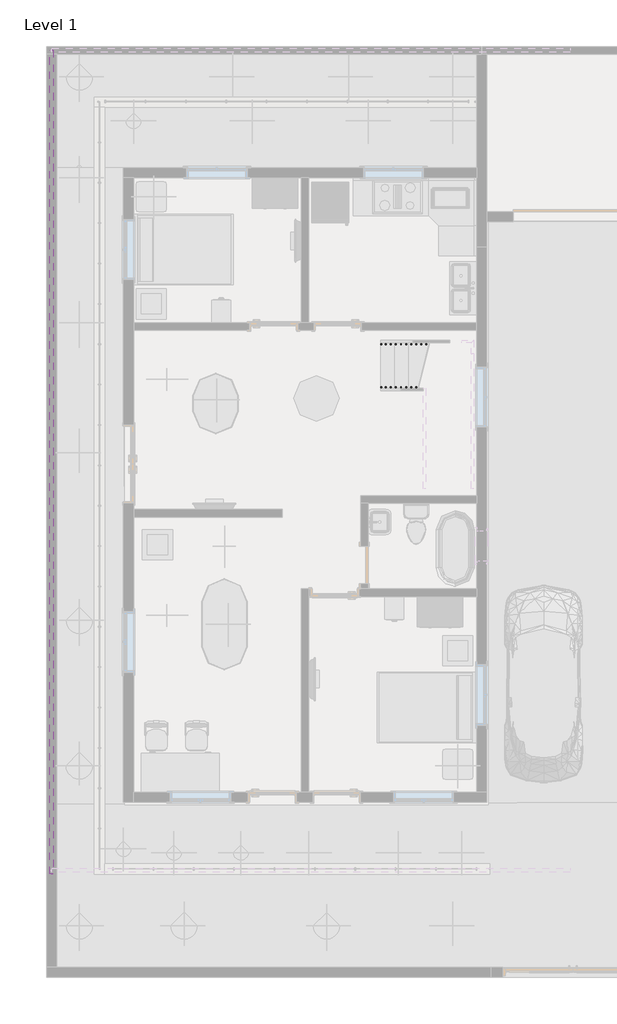
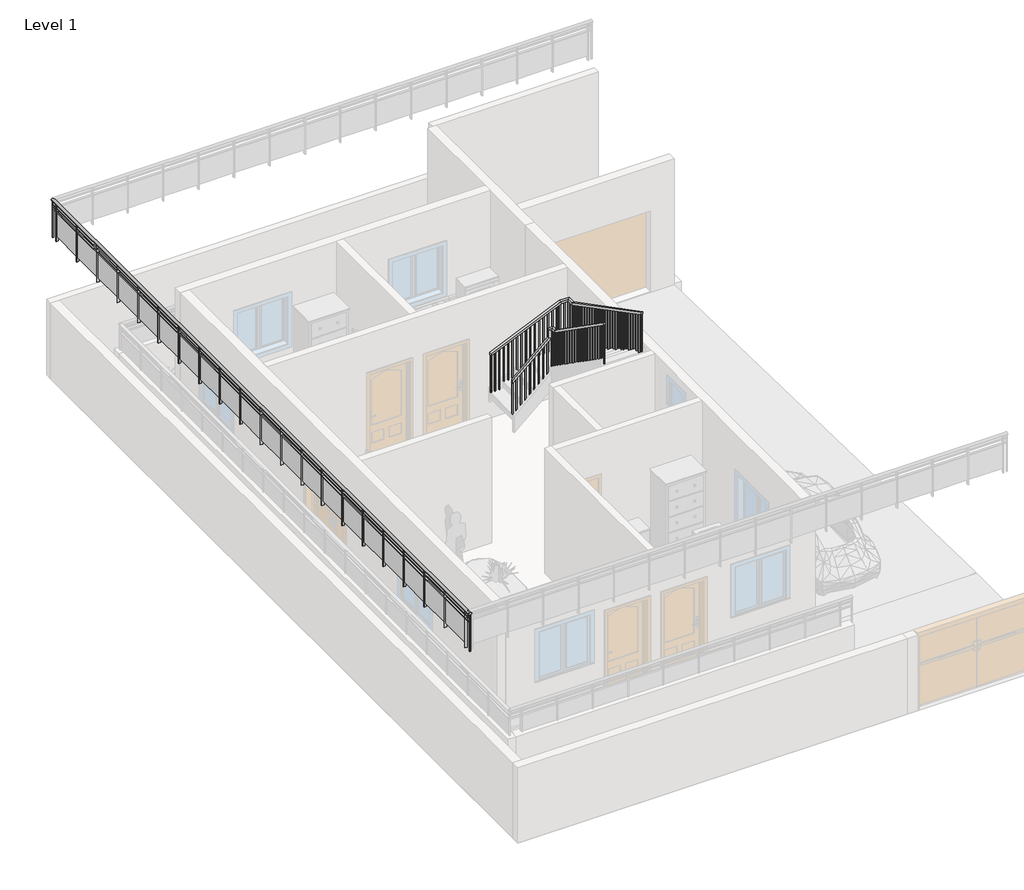
# One storey, part 3 of 5: 3 railings.
"""IFC4 building model written with IfcOpenShell, lengths in millimetres."""

from ifc_helpers import new_model, si_unit, point, frame, origin, place, context, project, spatial, polyline, ellipse_curve, trimmed, outline, extrude, faceted_brep, element, save
from ifc_brep_helpers import plane_surface, extruded_surface, advanced_brep

model = new_model("IFC4")

# Units and contexts
model_context = context("Model", 3, world=origin())
ifc_project = project(units=[si_unit("LENGTHUNIT", "METRE", prefix="MILLI")], contexts=[model_context])

# Site, building, storey
site = spatial("IfcSite", under=ifc_project)
building = spatial("IfcBuilding", under=site)
storey = spatial("IfcBuildingStorey", under=building, Name="Level 1", Elevation=0.0)

# Railings
placement = place(None, origin())
element("IfcRailing", 1, ObjectType="Glass Panel - Bottom Fill", at=placement, inside=storey, context=model_context, shape_type="SolidModel", body=[
    advanced_brep(
    [(-10998.0350785, 11610.9033005, 4267.2), (-11074.2350785, 11610.9033005, 4267.2), (-10998.0350785, -4975.2966995, 4267.2), (-11074.2350785, -4975.2966995, 4267.2)],
    [
        (0, 1, ellipse_curve(frame((-11036.1350785, 11610.9033005, 4267.2), z_axis=(0.0, 1.0, 0.0), x_axis=(-1.0, 0.0, 0.0)), 38.1, 28.575)),
        (1, 0, ellipse_curve(frame((-11036.1350785, 11610.9033005, 4267.2), z_axis=(0.0, 1.0, 0.0), x_axis=(-1.0, 0.0, 0.0)), 38.1, 28.575)),
        (2, 3, ellipse_curve(frame((-11036.1350785, -4975.2966995, 4267.2), z_axis=(0.0, -1.0, 0.0), x_axis=(-1.0, 0.0, 0.0)), 38.1, 28.575)),
        (3, 2, ellipse_curve(frame((-11036.1350785, -4975.2966995, 4267.2), z_axis=(0.0, -1.0, 0.0), x_axis=(-1.0, 0.0, 0.0)), 38.1, 28.575)),
        (0, 2),
        (3, 1),
    ],
    [
        plane_surface(frame((-11036.1350785, 11610.9033005, 4267.2), z_axis=(0.0, 1.0, 0.0), x_axis=(0.0, 0.0, -1.0))),
        plane_surface(frame((-11036.1350785, -4975.2966995, 4267.2), z_axis=(0.0, -1.0, 0.0), x_axis=(0.0, 0.0, -1.0))),
        extruded_surface(trimmed(ellipse_curve(frame((-11036.1350785, -4975.2966995, 4267.2), z_axis=(0.0, 1.0, 0.0), x_axis=(-1.0, 0.0, 0.0)), 38.1, 28.575), [point((-10998.0350785, -4975.2966995, 4267.2))], [point((-11074.2350785, -4975.2966995, 4267.2))], True, "CARTESIAN"), (0.0, 16586.2, 0.0), 16586.2),
        extruded_surface(trimmed(ellipse_curve(frame((-11036.1350785, -4975.2966995, 4267.2), z_axis=(0.0, 1.0, 0.0), x_axis=(-1.0, 0.0, 0.0)), 38.1, 28.575), [point((-11074.2350785, -4975.2966995, 4267.2))], [point((-10998.0350785, -4975.2966995, 4267.2))], True, "CARTESIAN"), (0.0, 16586.2, 0.0), 16586.2),
    ],
    [
        (0, [[1, 2]]),
        (1, [[3, 4]]),
        (2, [[-1, 5, -4, 6]]),
        (3, [[-2, -6, -3, -5]]),
    ],
),
    extrude(outline(polyline([(-11048.8350785, 11610.9033005), (-11023.4350785, 11610.9033005), (-11023.4350785, -4975.2966995), (-11048.8350785, -4975.2966995), (-11048.8350785, 11610.9033005)])), frame((0.0, 0.0, 4152.9), z_axis=(0.0, 0.0, 1.0), x_axis=(1.0, 0.0, 0.0)), (0.0, 0.0, 1.0), 25.4),
    extrude(outline(polyline([(-11048.8350785, 11610.9033005), (-11023.4350785, 11610.9033005), (-11023.4350785, -4975.2966995), (-11048.8350785, -4975.2966995), (-11048.8350785, 11610.9033005)])), frame((0.0, 0.0, 4051.3), z_axis=(0.0, 0.0, 1.0), x_axis=(1.0, 0.0, 0.0)), (0.0, 0.0, 1.0), 25.4),
    extrude(outline(polyline([(-11061.5350785, -4803.8466995), (-11010.7350785, -4803.8466995), (-11010.7350785, -4816.5466995), (-11061.5350785, -4816.5466995), (-11061.5350785, -4803.8466995)])), frame((0.0, 0.0, 3352.8), z_axis=(0.0, 0.0, 1.0), x_axis=(1.0, 0.0, 0.0)), (0.0, 0.0, 1.0), 885.6788223),
    extrude(outline(polyline([(-11029.5999215, -3997.3966995), (-11029.5999215, -4810.1966995), (-11035.9499215, -4810.1966995), (-11035.9499215, -3997.3966995), (-11029.5999215, -3997.3966995)])), frame((0.0, 0.0, 3454.4), z_axis=(0.0, 0.0, 1.0), x_axis=(1.0, 0.0, 0.0)), (0.0, 0.0, 1.0), 596.9),
    extrude(outline(polyline([(-11061.5350785, -3991.0466995), (-11010.7350785, -3991.0466995), (-11010.7350785, -4003.7466995), (-11061.5350785, -4003.7466995), (-11061.5350785, -3991.0466995)])), frame((0.0, 0.0, 3352.8), z_axis=(0.0, 0.0, 1.0), x_axis=(1.0, 0.0, 0.0)), (0.0, 0.0, 1.0), 885.6788223),
    extrude(outline(polyline([(-11029.5999215, -3184.5966995), (-11029.5999215, -3997.3966995), (-11035.9499215, -3997.3966995), (-11035.9499215, -3184.5966995), (-11029.5999215, -3184.5966995)])), frame((0.0, 0.0, 3454.4), z_axis=(0.0, 0.0, 1.0), x_axis=(1.0, 0.0, 0.0)), (0.0, 0.0, 1.0), 596.9),
    extrude(outline(polyline([(-11061.5350785, -3178.2466995), (-11010.7350785, -3178.2466995), (-11010.7350785, -3190.9466995), (-11061.5350785, -3190.9466995), (-11061.5350785, -3178.2466995)])), frame((0.0, 0.0, 3352.8), z_axis=(0.0, 0.0, 1.0), x_axis=(1.0, 0.0, 0.0)), (0.0, 0.0, 1.0), 885.6788223),
    extrude(outline(polyline([(-11029.5999215, -2371.7966995), (-11029.5999215, -3184.5966995), (-11035.9499215, -3184.5966995), (-11035.9499215, -2371.7966995), (-11029.5999215, -2371.7966995)])), frame((0.0, 0.0, 3454.4), z_axis=(0.0, 0.0, 1.0), x_axis=(1.0, 0.0, 0.0)), (0.0, 0.0, 1.0), 596.9),
    extrude(outline(polyline([(-11061.5350785, -2365.4466995), (-11010.7350785, -2365.4466995), (-11010.7350785, -2378.1466995), (-11061.5350785, -2378.1466995), (-11061.5350785, -2365.4466995)])), frame((0.0, 0.0, 3352.8), z_axis=(0.0, 0.0, 1.0), x_axis=(1.0, 0.0, 0.0)), (0.0, 0.0, 1.0), 885.6788223),
    extrude(outline(polyline([(-11029.5999215, -1558.9966995), (-11029.5999215, -2371.7966995), (-11035.9499215, -2371.7966995), (-11035.9499215, -1558.9966995), (-11029.5999215, -1558.9966995)])), frame((0.0, 0.0, 3454.4), z_axis=(0.0, 0.0, 1.0), x_axis=(1.0, 0.0, 0.0)), (0.0, 0.0, 1.0), 596.9),
    extrude(outline(polyline([(-11061.5350785, -1552.6466995), (-11010.7350785, -1552.6466995), (-11010.7350785, -1565.3466995), (-11061.5350785, -1565.3466995), (-11061.5350785, -1552.6466995)])), frame((0.0, 0.0, 3352.8), z_axis=(0.0, 0.0, 1.0), x_axis=(1.0, 0.0, 0.0)), (0.0, 0.0, 1.0), 885.6788223),
    extrude(outline(polyline([(-11029.5999215, -746.1966995), (-11029.5999215, -1558.9966995), (-11035.9499215, -1558.9966995), (-11035.9499215, -746.1966995), (-11029.5999215, -746.1966995)])), frame((0.0, 0.0, 3454.4), z_axis=(0.0, 0.0, 1.0), x_axis=(1.0, 0.0, 0.0)), (0.0, 0.0, 1.0), 596.9),
    extrude(outline(polyline([(-11061.5350785, -739.8466995), (-11010.7350785, -739.8466995), (-11010.7350785, -752.5466995), (-11061.5350785, -752.5466995), (-11061.5350785, -739.8466995)])), frame((0.0, 0.0, 3352.8), z_axis=(0.0, 0.0, 1.0), x_axis=(1.0, 0.0, 0.0)), (0.0, 0.0, 1.0), 885.6788223),
    extrude(outline(polyline([(-11029.5999215, 66.6033005), (-11029.5999215, -746.1966995), (-11035.9499215, -746.1966995), (-11035.9499215, 66.6033005), (-11029.5999215, 66.6033005)])), frame((0.0, 0.0, 3454.4), z_axis=(0.0, 0.0, 1.0), x_axis=(1.0, 0.0, 0.0)), (0.0, 0.0, 1.0), 596.9),
    extrude(outline(polyline([(-11061.5350785, 72.9533005), (-11010.7350785, 72.9533005), (-11010.7350785, 60.2533005), (-11061.5350785, 60.2533005), (-11061.5350785, 72.9533005)])), frame((0.0, 0.0, 3352.8), z_axis=(0.0, 0.0, 1.0), x_axis=(1.0, 0.0, 0.0)), (0.0, 0.0, 1.0), 885.6788223),
    extrude(outline(polyline([(-11029.5999215, 879.4033005), (-11029.5999215, 66.6033005), (-11035.9499215, 66.6033005), (-11035.9499215, 879.4033005), (-11029.5999215, 879.4033005)])), frame((0.0, 0.0, 3454.4), z_axis=(0.0, 0.0, 1.0), x_axis=(1.0, 0.0, 0.0)), (0.0, 0.0, 1.0), 596.9),
    extrude(outline(polyline([(-11061.5350785, 885.7533005), (-11010.7350785, 885.7533005), (-11010.7350785, 873.0533005), (-11061.5350785, 873.0533005), (-11061.5350785, 885.7533005)])), frame((0.0, 0.0, 3352.8), z_axis=(0.0, 0.0, 1.0), x_axis=(1.0, 0.0, 0.0)), (0.0, 0.0, 1.0), 885.6788223),
    extrude(outline(polyline([(-11029.5999215, 1692.2033005), (-11029.5999215, 879.4033005), (-11035.9499215, 879.4033005), (-11035.9499215, 1692.2033005), (-11029.5999215, 1692.2033005)])), frame((0.0, 0.0, 3454.4), z_axis=(0.0, 0.0, 1.0), x_axis=(1.0, 0.0, 0.0)), (0.0, 0.0, 1.0), 596.9),
    extrude(outline(polyline([(-11061.5350785, 1698.5533005), (-11010.7350785, 1698.5533005), (-11010.7350785, 1685.8533005), (-11061.5350785, 1685.8533005), (-11061.5350785, 1698.5533005)])), frame((0.0, 0.0, 3352.8), z_axis=(0.0, 0.0, 1.0), x_axis=(1.0, 0.0, 0.0)), (0.0, 0.0, 1.0), 885.6788223),
    extrude(outline(polyline([(-11029.5999215, 2505.0033005), (-11029.5999215, 1692.2033005), (-11035.9499215, 1692.2033005), (-11035.9499215, 2505.0033005), (-11029.5999215, 2505.0033005)])), frame((0.0, 0.0, 3454.4), z_axis=(0.0, 0.0, 1.0), x_axis=(1.0, 0.0, 0.0)), (0.0, 0.0, 1.0), 596.9),
    extrude(outline(polyline([(-11061.5350785, 2511.3533005), (-11010.7350785, 2511.3533005), (-11010.7350785, 2498.6533005), (-11061.5350785, 2498.6533005), (-11061.5350785, 2511.3533005)])), frame((0.0, 0.0, 3352.8), z_axis=(0.0, 0.0, 1.0), x_axis=(1.0, 0.0, 0.0)), (0.0, 0.0, 1.0), 885.6788223),
    extrude(outline(polyline([(-11029.5999215, 3317.8033005), (-11029.5999215, 2505.0033005), (-11035.9499215, 2505.0033005), (-11035.9499215, 3317.8033005), (-11029.5999215, 3317.8033005)])), frame((0.0, 0.0, 3454.4), z_axis=(0.0, 0.0, 1.0), x_axis=(1.0, 0.0, 0.0)), (0.0, 0.0, 1.0), 596.9),
    extrude(outline(polyline([(-11061.5350785, 3324.1533005), (-11010.7350785, 3324.1533005), (-11010.7350785, 3311.4533005), (-11061.5350785, 3311.4533005), (-11061.5350785, 3324.1533005)])), frame((0.0, 0.0, 3352.8), z_axis=(0.0, 0.0, 1.0), x_axis=(1.0, 0.0, 0.0)), (0.0, 0.0, 1.0), 885.6788223),
    extrude(outline(polyline([(-11029.5999215, 4130.6033005), (-11029.5999215, 3317.8033005), (-11035.9499215, 3317.8033005), (-11035.9499215, 4130.6033005), (-11029.5999215, 4130.6033005)])), frame((0.0, 0.0, 3454.4), z_axis=(0.0, 0.0, 1.0), x_axis=(1.0, 0.0, 0.0)), (0.0, 0.0, 1.0), 596.9),
    extrude(outline(polyline([(-11061.5350785, 4136.9533005), (-11010.7350785, 4136.9533005), (-11010.7350785, 4124.2533005), (-11061.5350785, 4124.2533005), (-11061.5350785, 4136.9533005)])), frame((0.0, 0.0, 3352.8), z_axis=(0.0, 0.0, 1.0), x_axis=(1.0, 0.0, 0.0)), (0.0, 0.0, 1.0), 885.6788223),
    extrude(outline(polyline([(-11029.5999215, 4943.4033005), (-11029.5999215, 4130.6033005), (-11035.9499215, 4130.6033005), (-11035.9499215, 4943.4033005), (-11029.5999215, 4943.4033005)])), frame((0.0, 0.0, 3454.4), z_axis=(0.0, 0.0, 1.0), x_axis=(1.0, 0.0, 0.0)), (0.0, 0.0, 1.0), 596.9),
    extrude(outline(polyline([(-11061.5350785, 4949.7533005), (-11010.7350785, 4949.7533005), (-11010.7350785, 4937.0533005), (-11061.5350785, 4937.0533005), (-11061.5350785, 4949.7533005)])), frame((0.0, 0.0, 3352.8), z_axis=(0.0, 0.0, 1.0), x_axis=(1.0, 0.0, 0.0)), (0.0, 0.0, 1.0), 885.6788223),
    extrude(outline(polyline([(-11029.5999215, 5756.2033005), (-11029.5999215, 4943.4033005), (-11035.9499215, 4943.4033005), (-11035.9499215, 5756.2033005), (-11029.5999215, 5756.2033005)])), frame((0.0, 0.0, 3454.4), z_axis=(0.0, 0.0, 1.0), x_axis=(1.0, 0.0, 0.0)), (0.0, 0.0, 1.0), 596.9),
    extrude(outline(polyline([(-11061.5350785, 5762.5533005), (-11010.7350785, 5762.5533005), (-11010.7350785, 5749.8533005), (-11061.5350785, 5749.8533005), (-11061.5350785, 5762.5533005)])), frame((0.0, 0.0, 3352.8), z_axis=(0.0, 0.0, 1.0), x_axis=(1.0, 0.0, 0.0)), (0.0, 0.0, 1.0), 885.6788223),
    extrude(outline(polyline([(-11029.5999215, 6569.0033005), (-11029.5999215, 5756.2033005), (-11035.9499215, 5756.2033005), (-11035.9499215, 6569.0033005), (-11029.5999215, 6569.0033005)])), frame((0.0, 0.0, 3454.4), z_axis=(0.0, 0.0, 1.0), x_axis=(1.0, 0.0, 0.0)), (0.0, 0.0, 1.0), 596.9),
    extrude(outline(polyline([(-11061.5350785, 6575.3533005), (-11010.7350785, 6575.3533005), (-11010.7350785, 6562.6533005), (-11061.5350785, 6562.6533005), (-11061.5350785, 6575.3533005)])), frame((0.0, 0.0, 3352.8), z_axis=(0.0, 0.0, 1.0), x_axis=(1.0, 0.0, 0.0)), (0.0, 0.0, 1.0), 885.6788223),
    extrude(outline(polyline([(-11029.5999215, 7381.8033005), (-11029.5999215, 6569.0033005), (-11035.9499215, 6569.0033005), (-11035.9499215, 7381.8033005), (-11029.5999215, 7381.8033005)])), frame((0.0, 0.0, 3454.4), z_axis=(0.0, 0.0, 1.0), x_axis=(1.0, 0.0, 0.0)), (0.0, 0.0, 1.0), 596.9),
    extrude(outline(polyline([(-11061.5350785, 7388.1533005), (-11010.7350785, 7388.1533005), (-11010.7350785, 7375.4533005), (-11061.5350785, 7375.4533005), (-11061.5350785, 7388.1533005)])), frame((0.0, 0.0, 3352.8), z_axis=(0.0, 0.0, 1.0), x_axis=(1.0, 0.0, 0.0)), (0.0, 0.0, 1.0), 885.6788223),
    extrude(outline(polyline([(-11029.5999215, 8194.6033005), (-11029.5999215, 7381.8033005), (-11035.9499215, 7381.8033005), (-11035.9499215, 8194.6033005), (-11029.5999215, 8194.6033005)])), frame((0.0, 0.0, 3454.4), z_axis=(0.0, 0.0, 1.0), x_axis=(1.0, 0.0, 0.0)), (0.0, 0.0, 1.0), 596.9),
    extrude(outline(polyline([(-11061.5350785, 8200.9533005), (-11010.7350785, 8200.9533005), (-11010.7350785, 8188.2533005), (-11061.5350785, 8188.2533005), (-11061.5350785, 8200.9533005)])), frame((0.0, 0.0, 3352.8), z_axis=(0.0, 0.0, 1.0), x_axis=(1.0, 0.0, 0.0)), (0.0, 0.0, 1.0), 885.6788223),
    extrude(outline(polyline([(-11029.5999215, 9007.4033005), (-11029.5999215, 8194.6033005), (-11035.9499215, 8194.6033005), (-11035.9499215, 9007.4033005), (-11029.5999215, 9007.4033005)])), frame((0.0, 0.0, 3454.4), z_axis=(0.0, 0.0, 1.0), x_axis=(1.0, 0.0, 0.0)), (0.0, 0.0, 1.0), 596.9),
    extrude(outline(polyline([(-11061.5350785, 9013.7533005), (-11010.7350785, 9013.7533005), (-11010.7350785, 9001.0533005), (-11061.5350785, 9001.0533005), (-11061.5350785, 9013.7533005)])), frame((0.0, 0.0, 3352.8), z_axis=(0.0, 0.0, 1.0), x_axis=(1.0, 0.0, 0.0)), (0.0, 0.0, 1.0), 885.6788223),
    extrude(outline(polyline([(-11029.5999215, 9820.2033005), (-11029.5999215, 9007.4033005), (-11035.9499215, 9007.4033005), (-11035.9499215, 9820.2033005), (-11029.5999215, 9820.2033005)])), frame((0.0, 0.0, 3454.4), z_axis=(0.0, 0.0, 1.0), x_axis=(1.0, 0.0, 0.0)), (0.0, 0.0, 1.0), 596.9),
    extrude(outline(polyline([(-11061.5350785, 9826.5533005), (-11010.7350785, 9826.5533005), (-11010.7350785, 9813.8533005), (-11061.5350785, 9813.8533005), (-11061.5350785, 9826.5533005)])), frame((0.0, 0.0, 3352.8), z_axis=(0.0, 0.0, 1.0), x_axis=(1.0, 0.0, 0.0)), (0.0, 0.0, 1.0), 885.6788223),
    extrude(outline(polyline([(-11029.5999215, 10633.0033005), (-11029.5999215, 9820.2033005), (-11035.9499215, 9820.2033005), (-11035.9499215, 10633.0033005), (-11029.5999215, 10633.0033005)])), frame((0.0, 0.0, 3454.4), z_axis=(0.0, 0.0, 1.0), x_axis=(1.0, 0.0, 0.0)), (0.0, 0.0, 1.0), 596.9),
    extrude(outline(polyline([(-11061.5350785, 10639.3533005), (-11010.7350785, 10639.3533005), (-11010.7350785, 10626.6533005), (-11061.5350785, 10626.6533005), (-11061.5350785, 10639.3533005)])), frame((0.0, 0.0, 3352.8), z_axis=(0.0, 0.0, 1.0), x_axis=(1.0, 0.0, 0.0)), (0.0, 0.0, 1.0), 885.6788223),
    extrude(outline(polyline([(-11029.5999215, 11445.8033005), (-11029.5999215, 10633.0033005), (-11035.9499215, 10633.0033005), (-11035.9499215, 11445.8033005), (-11029.5999215, 11445.8033005)])), frame((0.0, 0.0, 3454.4), z_axis=(0.0, 0.0, 1.0), x_axis=(1.0, 0.0, 0.0)), (0.0, 0.0, 1.0), 596.9),
    extrude(outline(polyline([(-11061.5350785, 11452.1533005), (-11010.7350785, 11452.1533005), (-11010.7350785, 11439.4533005), (-11061.5350785, 11439.4533005), (-11061.5350785, 11452.1533005)])), frame((0.0, 0.0, 3352.8), z_axis=(0.0, 0.0, 1.0), x_axis=(1.0, 0.0, 0.0)), (0.0, 0.0, 1.0), 885.6788223),
    extrude(outline(polyline([(-11045.6600785, -4962.5966995), (-11026.6100785, -4962.5966995), (-11026.6100785, -4981.6466995), (-11045.6600785, -4981.6466995), (-11045.6600785, -4962.5966995)])), frame((0.0, 0.0, 3352.8), z_axis=(0.0, 0.0, 1.0), x_axis=(1.0, 0.0, 0.0)), (0.0, 0.0, 1.0), 885.6788223),
    extrude(outline(polyline([(-11045.6600785, 11617.2533005), (-11026.6100785, 11617.2533005), (-11026.6100785, 11598.2033005), (-11045.6600785, 11598.2033005), (-11045.6600785, 11617.2533005)])), frame((0.0, 0.0, 3352.8), z_axis=(0.0, 0.0, 1.0), x_axis=(1.0, 0.0, 0.0)), (0.0, 0.0, 1.0), 885.6788223),
])
element("IfcRailing", 2, ObjectType="Handrail - Rectangular", at=placement, inside=storey, context=model_context, shape_type="SolidModel", body=[
    faceted_brep([(-4406.7350785, 4854.5033005, 1682.9646102), (-4406.7350785, 4854.5033005, 1615.1075334), (-4406.7350785, 4803.7033005, 1615.1075334), (-4406.7350785, 4803.7033005, 1682.9646102), (-3578.998089, 4854.5033005, 2416.0047843), (-3528.198089, 4854.5033005, 2393.1359601), (-3528.198089, 4803.7033005, 2393.1359601), (-3578.998089, 4803.7033005, 2416.0047843), (-3578.998089, 4854.5033005, 2625.457216), (-3528.198089, 4854.5033005, 2574.657216), (-3528.198089, 4803.7033005, 2574.657216), (-3578.998089, 4803.7033005, 2625.457216), (-3451.998089, 4854.5033005, 2625.457216), (-3451.998089, 4854.5033005, 2574.657216), (-3502.798089, 4803.7033005, 2574.657216), (-3502.798089, 4803.7033005, 2625.457216), (-3451.998089, 4727.5033005, 2625.457216), (-3451.998089, 4711.4736647, 2574.657216), (-3502.798089, 4711.4736647, 2574.657216), (-3502.798089, 4727.5033005, 2625.457216), (-3451.998089, 2782.166311, 3988.8904479), (-3502.798089, 2782.166311, 3988.8904479), (-3502.798089, 2782.166311, 3926.8557166), (-3451.998089, 2782.166311, 3926.8557166)], [[[0, 1, 2, 3]], [[1, 0, 4, 5]], [[2, 1, 5, 6]], [[3, 2, 6, 7]], [[0, 3, 7, 4]], [[5, 4, 8, 9]], [[6, 5, 9, 10]], [[7, 6, 10, 11]], [[4, 7, 11, 8]], [[9, 8, 12, 13]], [[10, 9, 13, 14]], [[11, 10, 14, 15]], [[8, 11, 15, 12]], [[13, 12, 16, 17]], [[14, 13, 17, 18]], [[15, 14, 18, 19]], [[12, 15, 19, 16]], [[20, 21, 22, 23]], [[17, 16, 20, 23]], [[18, 17, 23, 22]], [[19, 18, 22, 21]], [[16, 19, 21, 20]]]),
    extrude(outline(polyline([(2787.5783005, 3923.0626019), (2806.6283005, 3909.7109805), (2806.6283005, 2878.6666667), (2787.5783005, 2878.6666667), (2787.5783005, 3923.0626019)])), frame((-3486.923089, 0.0, 0.0), z_axis=(1.0, 0.0, 0.0), x_axis=(0.0, 1.0, 0.0)), (0.0, 0.0, 1.0), 19.05),
    extrude(outline(polyline([(2889.1783005, 3851.8539542), (2908.2283005, 3838.5023328), (2908.2283005, 2878.6666667), (2889.1783005, 2878.6666667), (2889.1783005, 3851.8539542)])), frame((-3486.923089, 0.0, 0.0), z_axis=(1.0, 0.0, 0.0), x_axis=(0.0, 1.0, 0.0)), (0.0, 0.0, 1.0), 19.05),
    extrude(outline(polyline([(2990.7783005, 3780.7235858), (3009.8283005, 3767.3719643), (3009.8283005, 2878.6666667), (2990.7783005, 2878.6666667), (2990.7783005, 3780.7235858)])), frame((-3486.923089, 0.0, 0.0), z_axis=(1.0, 0.0, 0.0), x_axis=(0.0, 1.0, 0.0)), (0.0, 0.0, 1.0), 19.05),
    extrude(outline(polyline([(3092.3783005, 3709.514938), (3111.4283005, 3696.1633166), (3111.4283005, 2709.3333333), (3092.3783005, 2709.3333333), (3092.3783005, 3709.514938)])), frame((-3486.923089, 0.0, 0.0), z_axis=(1.0, 0.0, 0.0), x_axis=(0.0, 1.0, 0.0)), (0.0, 0.0, 1.0), 19.05),
    extrude(outline(polyline([(3193.9783005, 3638.3062903), (3213.0283005, 3624.9546689), (3213.0283005, 2709.3333333), (3193.9783005, 2709.3333333), (3193.9783005, 3638.3062903)])), frame((-3486.923089, 0.0, 0.0), z_axis=(1.0, 0.0, 0.0), x_axis=(0.0, 1.0, 0.0)), (0.0, 0.0, 1.0), 19.05),
    extrude(outline(polyline([(3295.5783005, 3567.0193634), (3314.6283005, 3553.667742), (3314.6283005, 2709.3333333), (3295.5783005, 2709.3333333), (3295.5783005, 3567.0193634)])), frame((-3486.923089, 0.0, 0.0), z_axis=(1.0, 0.0, 0.0), x_axis=(0.0, 1.0, 0.0)), (0.0, 0.0, 1.0), 19.05),
    extrude(outline(polyline([(3397.1783005, 3495.8889949), (3416.2283005, 3482.5373735), (3416.2283005, 2540.0), (3397.1783005, 2540.0), (3397.1783005, 3495.8889949)])), frame((-3486.923089, 0.0, 0.0), z_axis=(1.0, 0.0, 0.0), x_axis=(0.0, 1.0, 0.0)), (0.0, 0.0, 1.0), 19.05),
    extrude(outline(polyline([(3498.7783005, 3424.602068), (3517.8283005, 3411.2504466), (3517.8283005, 2540.0), (3498.7783005, 2540.0), (3498.7783005, 3424.602068)])), frame((-3486.923089, 0.0, 0.0), z_axis=(1.0, 0.0, 0.0), x_axis=(0.0, 1.0, 0.0)), (0.0, 0.0, 1.0), 19.05),
    extrude(outline(polyline([(3600.3783005, 3353.4716995), (3619.4283005, 3340.1200781), (3619.4283005, 2370.6666667), (3600.3783005, 2370.6666667), (3600.3783005, 3353.4716995)])), frame((-3486.923089, 0.0, 0.0), z_axis=(1.0, 0.0, 0.0), x_axis=(0.0, 1.0, 0.0)), (0.0, 0.0, 1.0), 19.05),
    extrude(outline(polyline([(3701.9783005, 3282.1847726), (3721.0283005, 3268.8331511), (3721.0283005, 2370.6666667), (3701.9783005, 2370.6666667), (3701.9783005, 3282.1847726)])), frame((-3486.923089, 0.0, 0.0), z_axis=(1.0, 0.0, 0.0), x_axis=(0.0, 1.0, 0.0)), (0.0, 0.0, 1.0), 19.05),
    extrude(outline(polyline([(3803.5783005, 3210.9761249), (3822.6283005, 3197.6245034), (3822.6283005, 2370.6666667), (3803.5783005, 2370.6666667), (3803.5783005, 3210.9761249)])), frame((-3486.923089, 0.0, 0.0), z_axis=(1.0, 0.0, 0.0), x_axis=(0.0, 1.0, 0.0)), (0.0, 0.0, 1.0), 19.05),
    extrude(outline(polyline([(3905.1783005, 3139.8457564), (3924.2283005, 3126.494135), (3924.2283005, 2201.3333333), (3905.1783005, 2201.3333333), (3905.1783005, 3139.8457564)])), frame((-3486.923089, 0.0, 0.0), z_axis=(1.0, 0.0, 0.0), x_axis=(0.0, 1.0, 0.0)), (0.0, 0.0, 1.0), 19.05),
    extrude(outline(polyline([(4006.7783005, 3068.5588295), (4025.8283005, 3055.207208), (4025.8283005, 2201.3333333), (4006.7783005, 2201.3333333), (4006.7783005, 3068.5588295)])), frame((-3486.923089, 0.0, 0.0), z_axis=(1.0, 0.0, 0.0), x_axis=(0.0, 1.0, 0.0)), (0.0, 0.0, 1.0), 19.05),
    extrude(outline(polyline([(4108.3783005, 2997.3501818), (4127.4283005, 2983.9985603), (4127.4283005, 2201.3333333), (4108.3783005, 2201.3333333), (4108.3783005, 2997.3501818)])), frame((-3486.923089, 0.0, 0.0), z_axis=(1.0, 0.0, 0.0), x_axis=(0.0, 1.0, 0.0)), (0.0, 0.0, 1.0), 19.05),
    extrude(outline(polyline([(4209.9783005, 2926.1415341), (4229.0283005, 2912.7899126), (4229.0283005, 2032.0), (4209.9783005, 2032.0), (4209.9783005, 2926.1415341)])), frame((-3486.923089, 0.0, 0.0), z_axis=(1.0, 0.0, 0.0), x_axis=(0.0, 1.0, 0.0)), (0.0, 0.0, 1.0), 19.05),
    extrude(outline(polyline([(4311.5783005, 2854.9328864), (4330.6283005, 2841.5812649), (4330.6283005, 2032.0), (4311.5783005, 2032.0), (4311.5783005, 2854.9328864)])), frame((-3486.923089, 0.0, 0.0), z_axis=(1.0, 0.0, 0.0), x_axis=(0.0, 1.0, 0.0)), (0.0, 0.0, 1.0), 19.05),
    extrude(outline(polyline([(4413.1783005, 2783.8025179), (4432.2283005, 2770.4508964), (4432.2283005, 1862.6666667), (4413.1783005, 1862.6666667), (4413.1783005, 2783.8025179)])), frame((-3486.923089, 0.0, 0.0), z_axis=(1.0, 0.0, 0.0), x_axis=(0.0, 1.0, 0.0)), (0.0, 0.0, 1.0), 19.05),
    extrude(outline(polyline([(4514.7783005, 2712.515591), (4533.8283005, 2699.1639695), (4533.8283005, 1862.6666667), (4514.7783005, 1862.6666667), (4514.7783005, 2712.515591)])), frame((-3486.923089, 0.0, 0.0), z_axis=(1.0, 0.0, 0.0), x_axis=(0.0, 1.0, 0.0)), (0.0, 0.0, 1.0), 19.05),
    extrude(outline(polyline([(4616.3783005, 2641.3852225), (4635.4283005, 2628.033601), (4635.4283005, 1693.3333333), (4616.3783005, 1693.3333333), (4616.3783005, 2641.3852225)])), frame((-3486.923089, 0.0, 0.0), z_axis=(1.0, 0.0, 0.0), x_axis=(0.0, 1.0, 0.0)), (0.0, 0.0, 1.0), 19.05),
    extrude(outline(polyline([(-3486.923089, 4737.0283005), (-3467.873089, 4737.0283005), (-3467.873089, 4717.9783005), (-3486.923089, 4717.9783005), (-3486.923089, 4737.0283005)])), frame((0.0, 0.0, 1693.3333333), z_axis=(0.0, 0.0, 1.0), x_axis=(1.0, 0.0, 0.0)), (0.0, 0.0, 1.0), 881.3238827),
    extrude(outline(polyline([(-3501.8600785, 4819.5783005), (-3501.8600785, 4838.6283005), (-3482.8100785, 4838.6283005), (-3482.8100785, 4819.5783005), (-3501.8600785, 4819.5783005)])), frame((0.0, 0.0, 1524.0), z_axis=(0.0, 0.0, 1.0), x_axis=(1.0, 0.0, 0.0)), (0.0, 0.0, 1.0), 1050.657216),
    extrude(outline(polyline([(2343.3548737, -3584.4100785), (2326.484279, -3603.4600785), (1354.6666667, -3603.4600785), (1354.6666667, -3584.4100785), (2343.3548737, -3584.4100785)])), frame((0.0, 4819.5783005, 0.0), z_axis=(0.0, 1.0, 0.0), x_axis=(0.0, 0.0, 1.0)), (0.0, 0.0, 1.0), 19.05),
    extrude(outline(polyline([(2253.3783684, -3686.0100785), (2236.5077736, -3705.0600785), (1185.3333333, -3705.0600785), (1185.3333333, -3686.0100785), (2253.3783684, -3686.0100785)])), frame((0.0, 4819.5783005, 0.0), z_axis=(0.0, 1.0, 0.0), x_axis=(0.0, 0.0, 1.0)), (0.0, 0.0, 1.0), 19.05),
    extrude(outline(polyline([(2163.401863, -3787.6100785), (2146.5312682, -3806.6600785), (1185.3333333, -3806.6600785), (1185.3333333, -3787.6100785), (2163.401863, -3787.6100785)])), frame((0.0, 4819.5783005, 0.0), z_axis=(0.0, 1.0, 0.0), x_axis=(0.0, 0.0, 1.0)), (0.0, 0.0, 1.0), 19.05),
    extrude(outline(polyline([(2073.4253576, -3889.2100785), (2056.5547629, -3908.2600785), (1016.0, -3908.2600785), (1016.0, -3889.2100785), (2073.4253576, -3889.2100785)])), frame((0.0, 4819.5783005, 0.0), z_axis=(0.0, 1.0, 0.0), x_axis=(0.0, 0.0, 1.0)), (0.0, 0.0, 1.0), 19.05),
    extrude(outline(polyline([(1983.4488522, -3990.8100785), (1966.5782575, -4009.8600785), (1016.0, -4009.8600785), (1016.0, -3990.8100785), (1983.4488522, -3990.8100785)])), frame((0.0, 4819.5783005, 0.0), z_axis=(0.0, 1.0, 0.0), x_axis=(0.0, 0.0, 1.0)), (0.0, 0.0, 1.0), 19.05),
    extrude(outline(polyline([(1893.4723469, -4092.4100785), (1876.6017521, -4111.4600785), (1016.0, -4111.4600785), (1016.0, -4092.4100785), (1893.4723469, -4092.4100785)])), frame((0.0, 4819.5783005, 0.0), z_axis=(0.0, 1.0, 0.0), x_axis=(0.0, 0.0, 1.0)), (0.0, 0.0, 1.0), 19.05),
    extrude(outline(polyline([(1803.4958415, -4194.0100785), (1786.6252467, -4213.0600785), (846.6666667, -4213.0600785), (846.6666667, -4194.0100785), (1803.4958415, -4194.0100785)])), frame((0.0, 4819.5783005, 0.0), z_axis=(0.0, 1.0, 0.0), x_axis=(0.0, 0.0, 1.0)), (0.0, 0.0, 1.0), 19.05),
    extrude(outline(polyline([(1713.5193361, -4295.6100785), (1696.6487414, -4314.6600785), (846.6666667, -4314.6600785), (846.6666667, -4295.6100785), (1713.5193361, -4295.6100785)])), frame((0.0, 4819.5783005, 0.0), z_axis=(0.0, 1.0, 0.0), x_axis=(0.0, 0.0, 1.0)), (0.0, 0.0, 1.0), 19.05),
    extrude(outline(polyline([(-3486.923089, 4838.6283005), (-3467.873089, 4838.6283005), (-3467.873089, 4819.5783005), (-3486.923089, 4819.5783005), (-3486.923089, 4838.6283005)])), frame((0.0, 0.0, 1524.0), z_axis=(0.0, 0.0, 1.0), x_axis=(1.0, 0.0, 0.0)), (0.0, 0.0, 1.0), 1050.657216),
    extrude(outline(polyline([(2782.166311, 3926.8557166), (2801.216311, 3913.5040952), (2801.216311, 2878.6666667), (2782.166311, 2878.6666667), (2782.166311, 3926.8557166)])), frame((-3486.923089, 0.0, 0.0), z_axis=(1.0, 0.0, 0.0), x_axis=(0.0, 1.0, 0.0)), (0.0, 0.0, 1.0), 19.05),
    extrude(outline(polyline([(1631.9781281, -4387.6850785), (1615.1075334, -4406.7350785), (846.6666667, -4406.7350785), (846.6666667, -4387.6850785), (1631.9781281, -4387.6850785)])), frame((0.0, 4819.5783005, 0.0), z_axis=(0.0, 1.0, 0.0), x_axis=(0.0, 0.0, 1.0)), (0.0, 0.0, 1.0), 19.05),
])
element("IfcRailing", 3, ObjectType="Handrail - Rectangular", at=placement, inside=storey, context=model_context, shape_type="SolidModel", body=[
    faceted_brep([(-4406.7350785, 5718.1033005, 1807.8545254), (-4406.7350785, 5718.1033005, 1752.3830665), (-4406.7350785, 5667.3033005, 1752.3830665), (-4406.7350785, 5667.3033005, 1807.8545254), (-2809.3820442, 5718.1033005, 2508.4571941), (-2798.7312582, 5718.1033005, 2457.6571941), (-2798.7312582, 5667.3033005, 2457.6571941), (-2809.3820442, 5667.3033005, 2508.4571941), (-2588.398089, 5718.1033005, 2508.4571941), (-2588.398089, 5718.1033005, 2457.6571941), (-2639.198089, 5667.3033005, 2457.6571941), (-2639.198089, 5667.3033005, 2508.4571941), (-2588.398089, 5527.9999566, 2508.4571941), (-2588.398089, 5515.5635621, 2457.6571941), (-2639.198089, 5515.5635621, 2457.6571941), (-2639.198089, 5527.9999566, 2508.4571941), (-2588.398089, 2782.166311, 3938.588476), (-2639.198089, 2782.166311, 3938.588476), (-2639.198089, 2782.166311, 3881.3111437), (-2588.398089, 2782.166311, 3881.3111437)], [[[0, 1, 2, 3]], [[1, 0, 4, 5]], [[2, 1, 5, 6]], [[3, 2, 6, 7]], [[0, 3, 7, 4]], [[5, 4, 8, 9]], [[6, 5, 9, 10]], [[7, 6, 10, 11]], [[4, 7, 11, 8]], [[9, 8, 12, 13]], [[10, 9, 13, 14]], [[11, 10, 14, 15]], [[8, 11, 15, 12]], [[16, 17, 18, 19]], [[13, 12, 16, 19]], [[14, 13, 19, 18]], [[15, 14, 18, 17]], [[12, 15, 17, 16]]]),
    extrude(outline(polyline([(2794.3249566, 3874.9727949), (2794.3249566, 2878.6666667), (2775.2749566, 2878.6666667), (2775.2749566, 3884.8947365), (2794.3249566, 3874.9727949)])), frame((-2623.323089, 0.0, 0.0), z_axis=(1.0, 0.0, 0.0), x_axis=(0.0, 1.0, 0.0)), (0.0, 0.0, 1.0), 19.05),
    extrude(outline(polyline([(2895.9249566, 3822.0557734), (2895.9249566, 2878.6666667), (2876.8749566, 2878.6666667), (2876.8749566, 3831.9777149), (2895.9249566, 3822.0557734)])), frame((-2623.323089, 0.0, 0.0), z_axis=(1.0, 0.0, 0.0), x_axis=(0.0, 1.0, 0.0)), (0.0, 0.0, 1.0), 19.05),
    extrude(outline(polyline([(2997.5249566, 3769.1444302), (2997.5249566, 2878.6666667), (2978.4749566, 2878.6666667), (2978.4749566, 3779.0663717), (2997.5249566, 3769.1444302)])), frame((-2623.323089, 0.0, 0.0), z_axis=(1.0, 0.0, 0.0), x_axis=(0.0, 1.0, 0.0)), (0.0, 0.0, 1.0), 19.05),
    extrude(outline(polyline([(3099.1249566, 3716.2217303), (3099.1249566, 2709.3333333), (3080.0749566, 2709.3333333), (3080.0749566, 3726.1436718), (3099.1249566, 3716.2217303)])), frame((-2623.323089, 0.0, 0.0), z_axis=(1.0, 0.0, 0.0), x_axis=(0.0, 1.0, 0.0)), (0.0, 0.0, 1.0), 19.05),
    extrude(outline(polyline([(3200.7249566, 3663.3047087), (3200.7249566, 2709.3333333), (3181.6749566, 2709.3333333), (3181.6749566, 3673.2266502), (3200.7249566, 3663.3047087)])), frame((-2623.323089, 0.0, 0.0), z_axis=(1.0, 0.0, 0.0), x_axis=(0.0, 1.0, 0.0)), (0.0, 0.0, 1.0), 19.05),
    extrude(outline(polyline([(3302.3249566, 3610.3933655), (3302.3249566, 2709.3333333), (3283.2749566, 2709.3333333), (3283.2749566, 3620.315307), (3302.3249566, 3610.3933655)])), frame((-2623.323089, 0.0, 0.0), z_axis=(1.0, 0.0, 0.0), x_axis=(0.0, 1.0, 0.0)), (0.0, 0.0, 1.0), 19.05),
    extrude(outline(polyline([(3403.9249566, 3557.4706656), (3403.9249566, 2540.0), (3384.8749566, 2540.0), (3384.8749566, 3567.3926071), (3403.9249566, 3557.4706656)])), frame((-2623.323089, 0.0, 0.0), z_axis=(1.0, 0.0, 0.0), x_axis=(0.0, 1.0, 0.0)), (0.0, 0.0, 1.0), 19.05),
    extrude(outline(polyline([(3505.5249566, 3504.553644), (3505.5249566, 2540.0), (3486.4749566, 2540.0), (3486.4749566, 3514.4755855), (3505.5249566, 3504.553644)])), frame((-2623.323089, 0.0, 0.0), z_axis=(1.0, 0.0, 0.0), x_axis=(0.0, 1.0, 0.0)), (0.0, 0.0, 1.0), 19.05),
    extrude(outline(polyline([(3607.1249566, 3451.6366224), (3607.1249566, 2540.0), (3588.0749566, 2540.0), (3588.0749566, 3461.558564), (3607.1249566, 3451.6366224)])), frame((-2623.323089, 0.0, 0.0), z_axis=(1.0, 0.0, 0.0), x_axis=(0.0, 1.0, 0.0)), (0.0, 0.0, 1.0), 19.05),
    extrude(outline(polyline([(3708.7249566, 3398.7196009), (3708.7249566, 2370.6666667), (3689.6749566, 2370.6666667), (3689.6749566, 3408.6415424), (3708.7249566, 3398.7196009)])), frame((-2623.323089, 0.0, 0.0), z_axis=(1.0, 0.0, 0.0), x_axis=(0.0, 1.0, 0.0)), (0.0, 0.0, 1.0), 19.05),
    extrude(outline(polyline([(3810.3249566, 3345.8025793), (3810.3249566, 2370.6666667), (3791.2749566, 2370.6666667), (3791.2749566, 3355.7245208), (3810.3249566, 3345.8025793)])), frame((-2623.323089, 0.0, 0.0), z_axis=(1.0, 0.0, 0.0), x_axis=(0.0, 1.0, 0.0)), (0.0, 0.0, 1.0), 19.05),
    extrude(outline(polyline([(3911.9249566, 3292.8912361), (3911.9249566, 2370.6666667), (3892.8749566, 2370.6666667), (3892.8749566, 3302.8131776), (3911.9249566, 3292.8912361)])), frame((-2623.323089, 0.0, 0.0), z_axis=(1.0, 0.0, 0.0), x_axis=(0.0, 1.0, 0.0)), (0.0, 0.0, 1.0), 19.05),
    extrude(outline(polyline([(4013.5249566, 3239.9742145), (4013.5249566, 2201.3333333), (3994.4749566, 2201.3333333), (3994.4749566, 3249.8961561), (4013.5249566, 3239.9742145)])), frame((-2623.323089, 0.0, 0.0), z_axis=(1.0, 0.0, 0.0), x_axis=(0.0, 1.0, 0.0)), (0.0, 0.0, 1.0), 19.05),
    extrude(outline(polyline([(4115.1249566, 3187.057193), (4115.1249566, 2201.3333333), (4096.0749566, 2201.3333333), (4096.0749566, 3196.9791345), (4115.1249566, 3187.057193)])), frame((-2623.323089, 0.0, 0.0), z_axis=(1.0, 0.0, 0.0), x_axis=(0.0, 1.0, 0.0)), (0.0, 0.0, 1.0), 19.05),
    extrude(outline(polyline([(4216.7249566, 3134.1401714), (4216.7249566, 2201.3333333), (4197.6749566, 2201.3333333), (4197.6749566, 3144.062113), (4216.7249566, 3134.1401714)])), frame((-2623.323089, 0.0, 0.0), z_axis=(1.0, 0.0, 0.0), x_axis=(0.0, 1.0, 0.0)), (0.0, 0.0, 1.0), 19.05),
    extrude(outline(polyline([(4318.3249566, 3081.2231498), (4318.3249566, 2032.0), (4299.2749566, 2032.0), (4299.2749566, 3091.1450914), (4318.3249566, 3081.2231498)])), frame((-2623.323089, 0.0, 0.0), z_axis=(1.0, 0.0, 0.0), x_axis=(0.0, 1.0, 0.0)), (0.0, 0.0, 1.0), 19.05),
    extrude(outline(polyline([(4419.9249566, 3028.3061283), (4419.9249566, 2032.0), (4400.8749566, 2032.0), (4400.8749566, 3038.2280698), (4419.9249566, 3028.3061283)])), frame((-2623.323089, 0.0, 0.0), z_axis=(1.0, 0.0, 0.0), x_axis=(0.0, 1.0, 0.0)), (0.0, 0.0, 1.0), 19.05),
    extrude(outline(polyline([(4521.5249566, 2975.3891067), (4521.5249566, 2032.0), (4502.4749566, 2032.0), (4502.4749566, 2985.3110483), (4521.5249566, 2975.3891067)])), frame((-2623.323089, 0.0, 0.0), z_axis=(1.0, 0.0, 0.0), x_axis=(0.0, 1.0, 0.0)), (0.0, 0.0, 1.0), 19.05),
    extrude(outline(polyline([(4623.1249566, 2922.4720852), (4623.1249566, 1862.6666667), (4604.0749566, 1862.6666667), (4604.0749566, 2932.3940267), (4623.1249566, 2922.4720852)])), frame((-2623.323089, 0.0, 0.0), z_axis=(1.0, 0.0, 0.0), x_axis=(0.0, 1.0, 0.0)), (0.0, 0.0, 1.0), 19.05),
    extrude(outline(polyline([(4724.7249566, 2869.5550636), (4724.7249566, 1862.6666667), (4705.6749566, 1862.6666667), (4705.6749566, 2879.4770051), (4724.7249566, 2869.5550636)])), frame((-2623.323089, 0.0, 0.0), z_axis=(1.0, 0.0, 0.0), x_axis=(0.0, 1.0, 0.0)), (0.0, 0.0, 1.0), 19.05),
    extrude(outline(polyline([(4826.3249566, 2816.638042), (4826.3249566, 1862.6666667), (4807.2749566, 1862.6666667), (4807.2749566, 2826.5599836), (4826.3249566, 2816.638042)])), frame((-2623.323089, 0.0, 0.0), z_axis=(1.0, 0.0, 0.0), x_axis=(0.0, 1.0, 0.0)), (0.0, 0.0, 1.0), 19.05),
    extrude(outline(polyline([(4927.9249566, 2763.7210205), (4927.9249566, 1693.3333333), (4908.8749566, 1693.3333333), (4908.8749566, 2773.642962), (4927.9249566, 2763.7210205)])), frame((-2623.323089, 0.0, 0.0), z_axis=(1.0, 0.0, 0.0), x_axis=(0.0, 1.0, 0.0)), (0.0, 0.0, 1.0), 19.05),
    extrude(outline(polyline([(5029.5249566, 2710.8039989), (5029.5249566, 1693.3333333), (5010.4749566, 1693.3333333), (5010.4749566, 2720.7259404), (5029.5249566, 2710.8039989)])), frame((-2623.323089, 0.0, 0.0), z_axis=(1.0, 0.0, 0.0), x_axis=(0.0, 1.0, 0.0)), (0.0, 0.0, 1.0), 19.05),
    extrude(outline(polyline([(5131.1249566, 2657.8869773), (5131.1249566, 1693.3333333), (5112.0749566, 1693.3333333), (5112.0749566, 2667.8089189), (5131.1249566, 2657.8869773)])), frame((-2623.323089, 0.0, 0.0), z_axis=(1.0, 0.0, 0.0), x_axis=(0.0, 1.0, 0.0)), (0.0, 0.0, 1.0), 19.05),
    extrude(outline(polyline([(5232.7249566, 2604.9699558), (5232.7249566, 1693.3333333), (5213.6749566, 1693.3333333), (5213.6749566, 2614.8918973), (5232.7249566, 2604.9699558)])), frame((-2623.323089, 0.0, 0.0), z_axis=(1.0, 0.0, 0.0), x_axis=(0.0, 1.0, 0.0)), (0.0, 0.0, 1.0), 19.05),
    extrude(outline(polyline([(5334.3249566, 2552.0529342), (5334.3249566, 1524.0), (5315.2749566, 1524.0), (5315.2749566, 2561.9748757), (5334.3249566, 2552.0529342)])), frame((-2623.323089, 0.0, 0.0), z_axis=(1.0, 0.0, 0.0), x_axis=(0.0, 1.0, 0.0)), (0.0, 0.0, 1.0), 19.05),
    extrude(outline(polyline([(5435.9249566, 2499.1359126), (5435.9249566, 1524.0), (5416.8749566, 1524.0), (5416.8749566, 2509.0578542), (5435.9249566, 2499.1359126)])), frame((-2623.323089, 0.0, 0.0), z_axis=(1.0, 0.0, 0.0), x_axis=(0.0, 1.0, 0.0)), (0.0, 0.0, 1.0), 19.05),
    extrude(outline(polyline([(-2604.273089, 5600.6283005), (-2604.273089, 5581.5783005), (-2623.323089, 5581.5783005), (-2623.323089, 5600.6283005), (-2604.273089, 5600.6283005)])), frame((0.0, 0.0, 1524.0), z_axis=(0.0, 0.0, 1.0), x_axis=(1.0, 0.0, 0.0)), (0.0, 0.0, 1.0), 933.6571941),
    extrude(outline(polyline([(-2717.3070442, 5702.2283005), (-2698.2570442, 5702.2283005), (-2698.2570442, 5683.1783005), (-2717.3070442, 5683.1783005), (-2717.3070442, 5702.2283005)])), frame((0.0, 0.0, 1524.0), z_axis=(0.0, 0.0, 1.0), x_axis=(1.0, 0.0, 0.0)), (0.0, 0.0, 1.0), 933.6571941),
    extrude(outline(polyline([(2416.6352411, -2892.2600785), (1524.0, -2892.2600785), (1524.0, -2873.2100785), (2424.9906144, -2873.2100785), (2416.6352411, -2892.2600785)])), frame((0.0, 5683.1783005, 0.0), z_axis=(0.0, 1.0, 0.0), x_axis=(0.0, 0.0, 1.0)), (0.0, 0.0, 1.0), 19.05),
    extrude(outline(polyline([(2372.0732504, -2993.8600785), (1524.0, -2993.8600785), (1524.0, -2974.8100785), (2380.4286236, -2974.8100785), (2372.0732504, -2993.8600785)])), frame((0.0, 5683.1783005, 0.0), z_axis=(0.0, 1.0, 0.0), x_axis=(0.0, 0.0, 1.0)), (0.0, 0.0, 1.0), 19.05),
    extrude(outline(polyline([(2327.5112596, -3095.4600785), (1354.6666667, -3095.4600785), (1354.6666667, -3076.4100785), (2335.8666329, -3076.4100785), (2327.5112596, -3095.4600785)])), frame((0.0, 5683.1783005, 0.0), z_axis=(0.0, 1.0, 0.0), x_axis=(0.0, 0.0, 1.0)), (0.0, 0.0, 1.0), 19.05),
    extrude(outline(polyline([(2282.9492689, -3197.0600785), (1354.6666667, -3197.0600785), (1354.6666667, -3178.0100785), (2291.3046421, -3178.0100785), (2282.9492689, -3197.0600785)])), frame((0.0, 5683.1783005, 0.0), z_axis=(0.0, 1.0, 0.0), x_axis=(0.0, 0.0, 1.0)), (0.0, 0.0, 1.0), 19.05),
    extrude(outline(polyline([(2238.3872781, -3298.6600785), (1354.6666667, -3298.6600785), (1354.6666667, -3279.6100785), (2246.7426514, -3279.6100785), (2238.3872781, -3298.6600785)])), frame((0.0, 5683.1783005, 0.0), z_axis=(0.0, 1.0, 0.0), x_axis=(0.0, 0.0, 1.0)), (0.0, 0.0, 1.0), 19.05),
    extrude(outline(polyline([(2193.8252874, -3400.2600785), (1354.6666667, -3400.2600785), (1354.6666667, -3381.2100785), (2202.1806606, -3381.2100785), (2193.8252874, -3400.2600785)])), frame((0.0, 5683.1783005, 0.0), z_axis=(0.0, 1.0, 0.0), x_axis=(0.0, 0.0, 1.0)), (0.0, 0.0, 1.0), 19.05),
    extrude(outline(polyline([(2149.2632966, -3501.8600785), (1185.3333333, -3501.8600785), (1185.3333333, -3482.8100785), (2157.6186699, -3482.8100785), (2149.2632966, -3501.8600785)])), frame((0.0, 5683.1783005, 0.0), z_axis=(0.0, 1.0, 0.0), x_axis=(0.0, 0.0, 1.0)), (0.0, 0.0, 1.0), 19.05),
    extrude(outline(polyline([(2104.7013059, -3603.4600785), (1185.3333333, -3603.4600785), (1185.3333333, -3584.4100785), (2113.0566791, -3584.4100785), (2104.7013059, -3603.4600785)])), frame((0.0, 5683.1783005, 0.0), z_axis=(0.0, 1.0, 0.0), x_axis=(0.0, 0.0, 1.0)), (0.0, 0.0, 1.0), 19.05),
    extrude(outline(polyline([(2060.1393151, -3705.0600785), (1185.3333333, -3705.0600785), (1185.3333333, -3686.0100785), (2068.4946884, -3686.0100785), (2060.1393151, -3705.0600785)])), frame((0.0, 5683.1783005, 0.0), z_axis=(0.0, 1.0, 0.0), x_axis=(0.0, 0.0, 1.0)), (0.0, 0.0, 1.0), 19.05),
    extrude(outline(polyline([(2015.5773244, -3806.6600785), (1185.3333333, -3806.6600785), (1185.3333333, -3787.6100785), (2023.9326976, -3787.6100785), (2015.5773244, -3806.6600785)])), frame((0.0, 5683.1783005, 0.0), z_axis=(0.0, 1.0, 0.0), x_axis=(0.0, 0.0, 1.0)), (0.0, 0.0, 1.0), 19.05),
    extrude(outline(polyline([(1971.0153336, -3908.2600785), (1016.0, -3908.2600785), (1016.0, -3889.2100785), (1979.3707069, -3889.2100785), (1971.0153336, -3908.2600785)])), frame((0.0, 5683.1783005, 0.0), z_axis=(0.0, 1.0, 0.0), x_axis=(0.0, 0.0, 1.0)), (0.0, 0.0, 1.0), 19.05),
    extrude(outline(polyline([(1926.4533429, -4009.8600785), (1016.0, -4009.8600785), (1016.0, -3990.8100785), (1934.8087161, -3990.8100785), (1926.4533429, -4009.8600785)])), frame((0.0, 5683.1783005, 0.0), z_axis=(0.0, 1.0, 0.0), x_axis=(0.0, 0.0, 1.0)), (0.0, 0.0, 1.0), 19.05),
    extrude(outline(polyline([(1881.8913521, -4111.4600785), (1016.0, -4111.4600785), (1016.0, -4092.4100785), (1890.2467254, -4092.4100785), (1881.8913521, -4111.4600785)])), frame((0.0, 5683.1783005, 0.0), z_axis=(0.0, 1.0, 0.0), x_axis=(0.0, 0.0, 1.0)), (0.0, 0.0, 1.0), 19.05),
    extrude(outline(polyline([(1837.3293614, -4213.0600785), (846.6666667, -4213.0600785), (846.6666667, -4194.0100785), (1845.6847346, -4194.0100785), (1837.3293614, -4213.0600785)])), frame((0.0, 5683.1783005, 0.0), z_axis=(0.0, 1.0, 0.0), x_axis=(0.0, 0.0, 1.0)), (0.0, 0.0, 1.0), 19.05),
    extrude(outline(polyline([(1792.7673706, -4314.6600785), (846.6666667, -4314.6600785), (846.6666667, -4295.6100785), (1801.1227439, -4295.6100785), (1792.7673706, -4314.6600785)])), frame((0.0, 5683.1783005, 0.0), z_axis=(0.0, 1.0, 0.0), x_axis=(0.0, 0.0, 1.0)), (0.0, 0.0, 1.0), 19.05),
    extrude(outline(polyline([(-2604.273089, 5537.5249566), (-2604.273089, 5518.4749566), (-2623.323089, 5518.4749566), (-2623.323089, 5537.5249566), (-2604.273089, 5537.5249566)])), frame((0.0, 0.0, 1524.0), z_axis=(0.0, 0.0, 1.0), x_axis=(1.0, 0.0, 0.0)), (0.0, 0.0, 1.0), 933.6571941),
    extrude(outline(polyline([(-2623.323089, 5702.2283005), (-2604.273089, 5702.2283005), (-2604.273089, 5683.1783005), (-2623.323089, 5683.1783005), (-2623.323089, 5702.2283005)])), frame((0.0, 0.0, 1524.0), z_axis=(0.0, 0.0, 1.0), x_axis=(1.0, 0.0, 0.0)), (0.0, 0.0, 1.0), 933.6571941),
    extrude(outline(polyline([(2448.8080486, -2818.9070442), (1524.0, -2818.9070442), (1524.0, -2799.8570442), (2457.1634218, -2799.8570442), (2448.8080486, -2818.9070442)])), frame((0.0, 5683.1783005, 0.0), z_axis=(0.0, 1.0, 0.0), x_axis=(0.0, 0.0, 1.0)), (0.0, 0.0, 1.0), 19.05),
    extrude(outline(polyline([(2801.216311, 3871.3892021), (2801.216311, 2878.6666667), (2782.166311, 2878.6666667), (2782.166311, 3881.3111437), (2801.216311, 3871.3892021)])), frame((-2623.323089, 0.0, 0.0), z_axis=(1.0, 0.0, 0.0), x_axis=(0.0, 1.0, 0.0)), (0.0, 0.0, 1.0), 19.05),
    extrude(outline(polyline([(1752.3830665, -4406.7350785), (846.6666667, -4406.7350785), (846.6666667, -4387.6850785), (1760.7384398, -4387.6850785), (1752.3830665, -4406.7350785)])), frame((0.0, 5683.1783005, 0.0), z_axis=(0.0, 1.0, 0.0), x_axis=(0.0, 0.0, 1.0)), (0.0, 0.0, 1.0), 19.05),
])

save(model, "model.ifc")

# Revit data of these elements
# Type "Glass Panel - Bottom Fill"
#   Assembly Code = "C2010400"
#   built-in parameter 1008612 = 0.0416667 (stored number, unit not read)
#   built-in parameter 1008611 = 0.0416667 (stored number, unit not read)
#   built-in parameter 1008609 = 0.333333 (stored number, unit not read)
#   built-in parameter 1008604 = 0.166667 (stored number, unit not read)
#   built-in parameter 1008603 = 0.166667 (stored number, unit not read)
#   Railing Height = 3' - 0"
#   built-in parameter 1008630 = 2
#   built-in parameter 1008610 = 2
#   built-in parameter 1008618 = Baluster - Square : 3/4"
# Type "Handrail - Rectangular"
#   Assembly Code = "C2010400"
#   built-in parameter 1008612 = 0.0416667 (stored number, unit not read)
#   built-in parameter 1008611 = 0.0416667 (stored number, unit not read)
#   built-in parameter 1008609 = 0.333333 (stored number, unit not read)
#   built-in parameter 1008604 = 0.166667 (stored number, unit not read)
#   built-in parameter 1008603 = 0.166667 (stored number, unit not read)
#   Railing Height = 3' - 0"
#   built-in parameter 1008630 = 2
#   built-in parameter 1008610 = 2
#   built-in parameter 1008618 = Baluster - Square : 3/4"
# Element 1 (IfcRailing, "Glass Panel - Bottom Fill")
#   built-in parameter 1008621 = 11 (stored number, unit not read)
#   Phase Created = New Construction
#   Materials on its faces: "Glass"
# Elements 2, 3 (IfcRailing, "Handrail - Rectangular")
#   Phase Created = New Construction
# Materials
#   "Glass": class "Glass", colour RGB 0 128 192, transparency 0.75, Description = "Soda Lime Glass", Cost = 0
